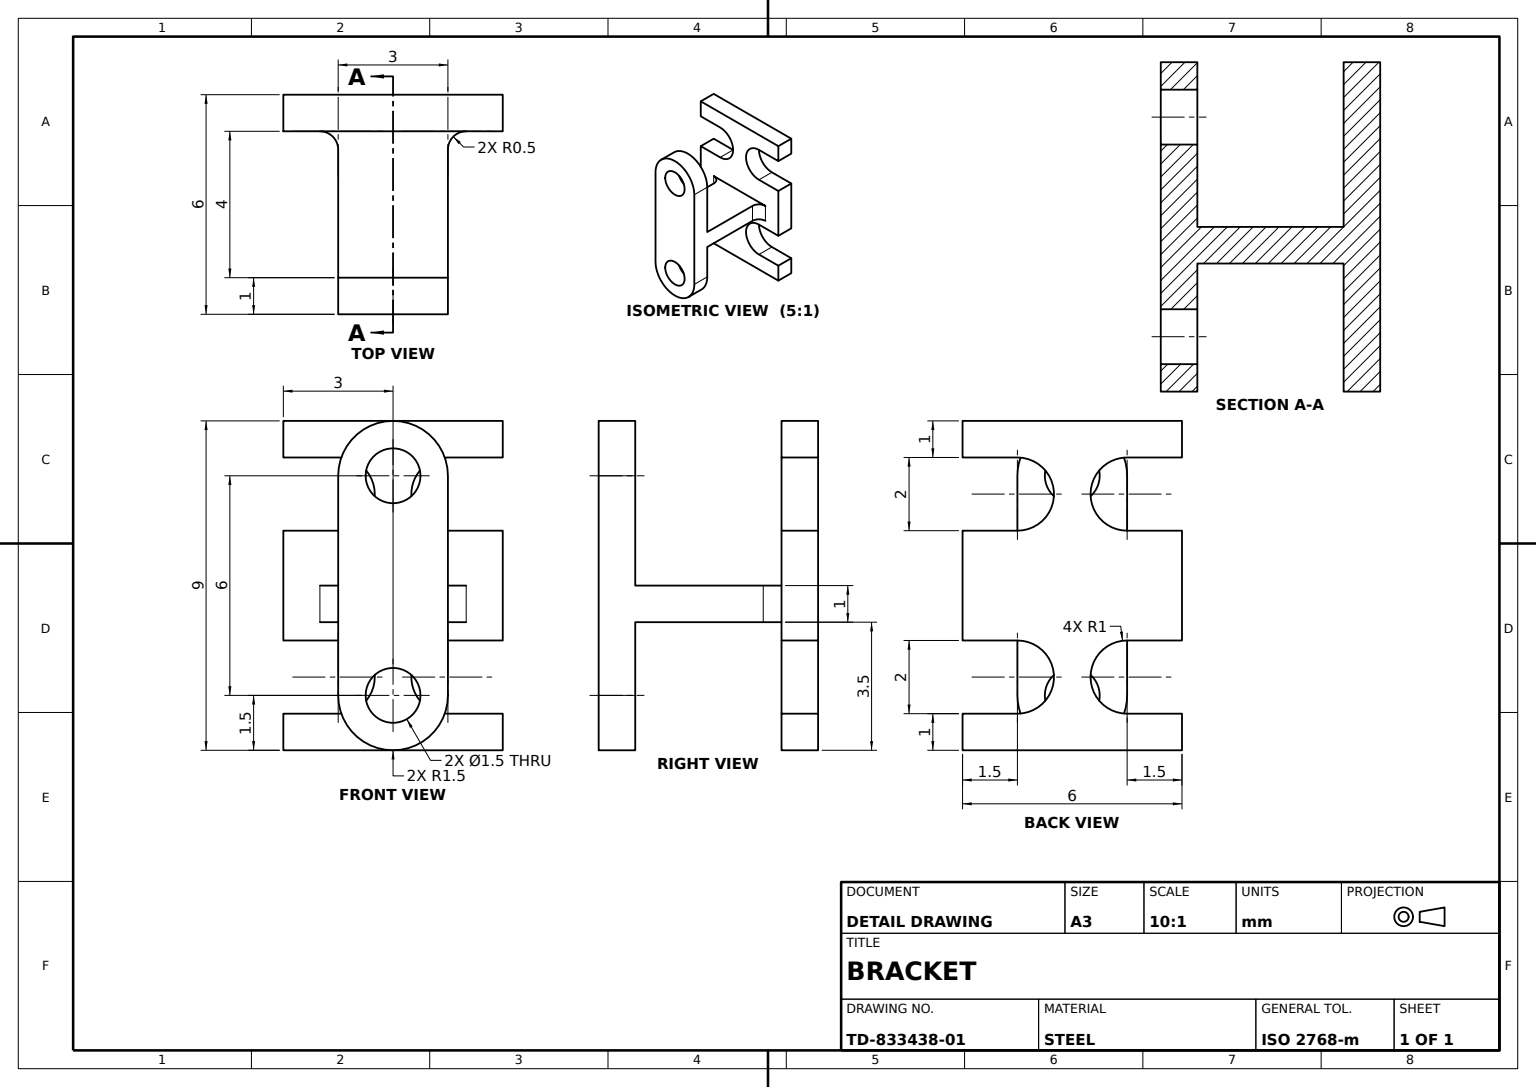
SolidWorks part; units mm, degrees
material "Plain Carbon Steel"
ref_plane "Front Plane" through (0, 0, 0) normal (0, 0, 1) x (1, 0, 0)
ref_plane "Top Plane" through (0, 0, 0) normal (0, 1, 0) x (1, 0, 0)
ref_plane "Right Plane" through (0, 0, 0) normal (1, 0, 0) x (0, 0, -1)
sketch "Base Plate Sketch" plane through (0, 0, 0) normal (0, 0, 1) x (1, 0, 0)
  line L1 (-3, 3) -> (3, 3)
  line L2 (-3, 3) -> (-3, -3)
  line L3 (-3, -3) -> (3, -3)
  line L4 (3, 3) -> (3, -3)
  line L5 (-3, 3) -> (3, -3) construction
  line L6 (-3, -3) -> (3, 3) construction
  point P0 (0, 0)
  dimension "D1" = 6
  dimension "D2" = 6
extrude "Base Plate" add sketch "Base Plate Sketch" against normal blind 1
sketch "Upper Pad Sketch" plane through (0, 3, 0) normal (0, 1, 0) x (1, 0, 0)
  line L1 (-3, 1) -> (3, 1)
  line L2 (-3, 1) -> (-3, 0)
  line L3 (-3, 0) -> (3, 0)
  line L4 (3, 1) -> (3, 0)
extrude "Upper Pad" add sketch "Upper Pad Sketch" along normal blind 1.5
sketch "Lower Pad Sketch" plane through (0, -3, 0) normal (0, -1, 0) x (1, 0, 0)
  line L1 (-3, 0) -> (3, 0)
  line L2 (-3, 0) -> (-3, -1)
  line L3 (-3, -1) -> (3, -1)
  line L4 (3, 0) -> (3, -1)
extrude "Lower Pad" add sketch "Lower Pad Sketch" along normal blind 1.5
sketch "Notch Cut Sketch" plane through (0, 0, 0) normal (0, 0, 1) x (1, 0, 0)
  line L0 (0, 4.5) -> (0, -4.5) construction
  line L1 (-3, 4.5) -> (3, 4.5) construction
  line L2 (3, -4.5) -> (-3, -4.5) construction
  line L3 (-3, 4.5) -> (-3, -4.5) construction
  line L4 (-1.5, 3.5) -> (-3, 3.5)
  line L5 (-1.5, 1.5) -> (-3, 1.5)
  line L6 (-3, 1.5) -> (-3, 3.5)
  line L7 (-3, 0) -> (3, 0) construction
  line L8 (3, -4.5) -> (3, 4.5) construction
  line L9 (1.5, 3.5) -> (3, 3.5)
  line L10 (1.5, 1.5) -> (3, 1.5)
  line L11 (3, 1.5) -> (3, 3.5)
  line L12 (3, -1.5) -> (3, -3.5)
  line L13 (1.5, -1.5) -> (3, -1.5)
  line L14 (1.5, -3.5) -> (3, -3.5)
  line L15 (-1.5, -1.5) -> (-3, -1.5)
  line L16 (-3, -1.5) -> (-3, -3.5)
  line L17 (-1.5, -3.5) -> (-3, -3.5)
  arc A0 (-1.5, 1.5) -> (-1.5, 3.5) centre (-1.5, 2.5) ccw
  arc A1 (1.5, 1.5) -> (1.5, 3.5) centre (1.5, 2.5) cw
  arc A2 (1.5, -1.5) -> (1.5, -3.5) centre (1.5, -2.5) ccw
  arc A3 (-1.5, -1.5) -> (-1.5, -3.5) centre (-1.5, -2.5) cw
  dimension "D1" = 2
  dimension "D2" = 2
  dimension "D3" = 1.5
  dimension "D4" = 3
extrude "Notch Cuts" cut sketch "Notch Cut Sketch" against normal blind 1.5
sketch "Stem Sketch" plane through (0, 0, 0) normal (0, 0, 1) x (1, 0, 0)
  line L0 (-1.5, 0) -> (1.5, 0)
  line L1 (1.5, 0) -> (1.5, -1)
  line L2 (1.5, -1) -> (-1.5, -1)
  line L3 (-1.5, -1) -> (-1.5, 0)
  point P4 (0, 0)
  dimension "D1" = 1
  dimension "D2" = 3
extrude "Stem 1x3" add sketch "Stem Sketch" along normal blind 4
fillet "Stem Fillet R0.5 A" radius 0.5 1 edges at (1.5, -0.5, 0)
fillet "Stem Fillet R0.5 B" radius 0.5 1 edges at (-1.5, -0.5, 0)
sketch "Lug Plate Sketch" plane through (0, 0, 4) normal (0, 0, 1) x (1, 0, 0)
  line L0 (0, 3) -> (0, -3) construction
  line L4 (1.5, 3) -> (1.5, -3)
  line L5 (-1.5, 3) -> (-1.5, -3)
  arc A2 (1.5, 3) -> (-1.5, 3) centre (0, 3) ccw
  arc A3 (-1.5, -3) -> (1.5, -3) centre (0, -3) ccw
  circle A4 centre (0, 3) radius 0.75
  circle A5 centre (0, -3) radius 0.75
  point P2 (0, 0)
  point P8 (0, 4.5)
  point P9 (0, -4.5)
  dimension "D2" = 1.5
  dimension "D3" = 1.5
  dimension "D4" = 1.5
  dimension "D1" = 9
extrude "Lug Plate" add sketch "Lug Plate Sketch" along normal blind 1
